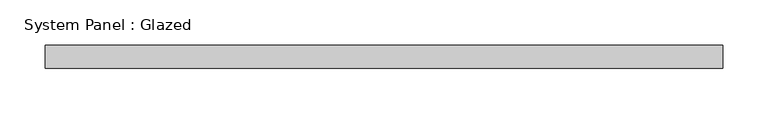
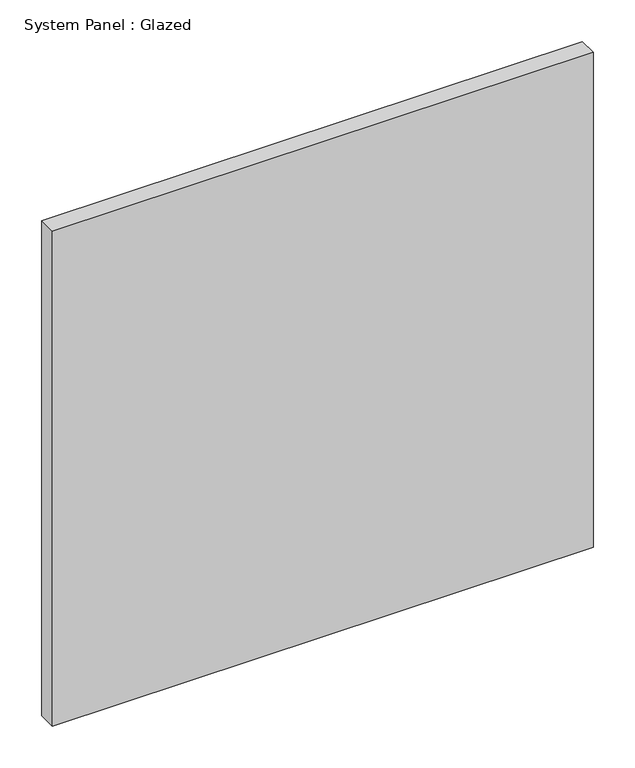
"""IFC4 building model written with IfcOpenShell, lengths in millimetres: plate geometry, System Panel : Glazed."""

from ifc_helpers import new_model, si_unit, origin, origin_with_axes, place, context, project, spatial, polyline, outline, extrude, source, transform, mapped, element, save


def system_panel_glazed_ecd9048c(model_context):
    return source(origin(), model_context, "Body", "SweptSolid", [
        extrude(outline(polyline([(374.65, 19.05), (-374.65, 19.05), (-374.65, 44.45), (374.65, 44.45), (374.65, 19.05)])), origin_with_axes(), (0.0, 0.0, 1.0), 725.1381029),
    ])


if __name__ == "__main__":
    model = new_model("IFC4")
    model_context = context("Model", 3, world=origin())
    ifc_project = project(units=[si_unit("LENGTHUNIT", "METRE", prefix="MILLI")], contexts=[model_context])
    site = spatial("IfcSite", under=ifc_project)
    building = spatial("IfcBuilding", under=site)
    placement = place(None, origin())
    system_panel_glazed_shape = system_panel_glazed_ecd9048c(model_context)
    element("IfcPlate", 1, ObjectType="System Panel : Glazed", at=placement, inside=building, context=model_context, shape_type="MappedRepresentation", body=[
        mapped(system_panel_glazed_shape, transform((0.0, 0.0, 0.0), x_axis=(1.0, 0.0, 0.0), y_axis=(0.0, 1.0, 0.0), z_axis=(0.0, 0.0, 1.0))),
    ])
    save(model, "model.ifc")

# Revit data of these elements
# Type "System Panel : Glazed"
#   Construction Type Id = "GSP4R"
#   Analytic Construction = "1/8 in Pilkington single glazing"
#   Visual Light Transmittance = 0.9
#   Solar Heat Gain Coefficient = 0.86
#   Heat Transfer Coefficient (U) = 1.18115 BTU/(h·ft²·°F)
#   Define Thermal Properties by = 1
# Element 1 (IfcPlate, "System Panel : Glazed")
#   Materials on its faces: "Glass"
# Materials
#   "Glass": class "Glass", colour RGB 0 128 192, transparency 0.75, Description = "Soda Lime Glass", Cost = 0
